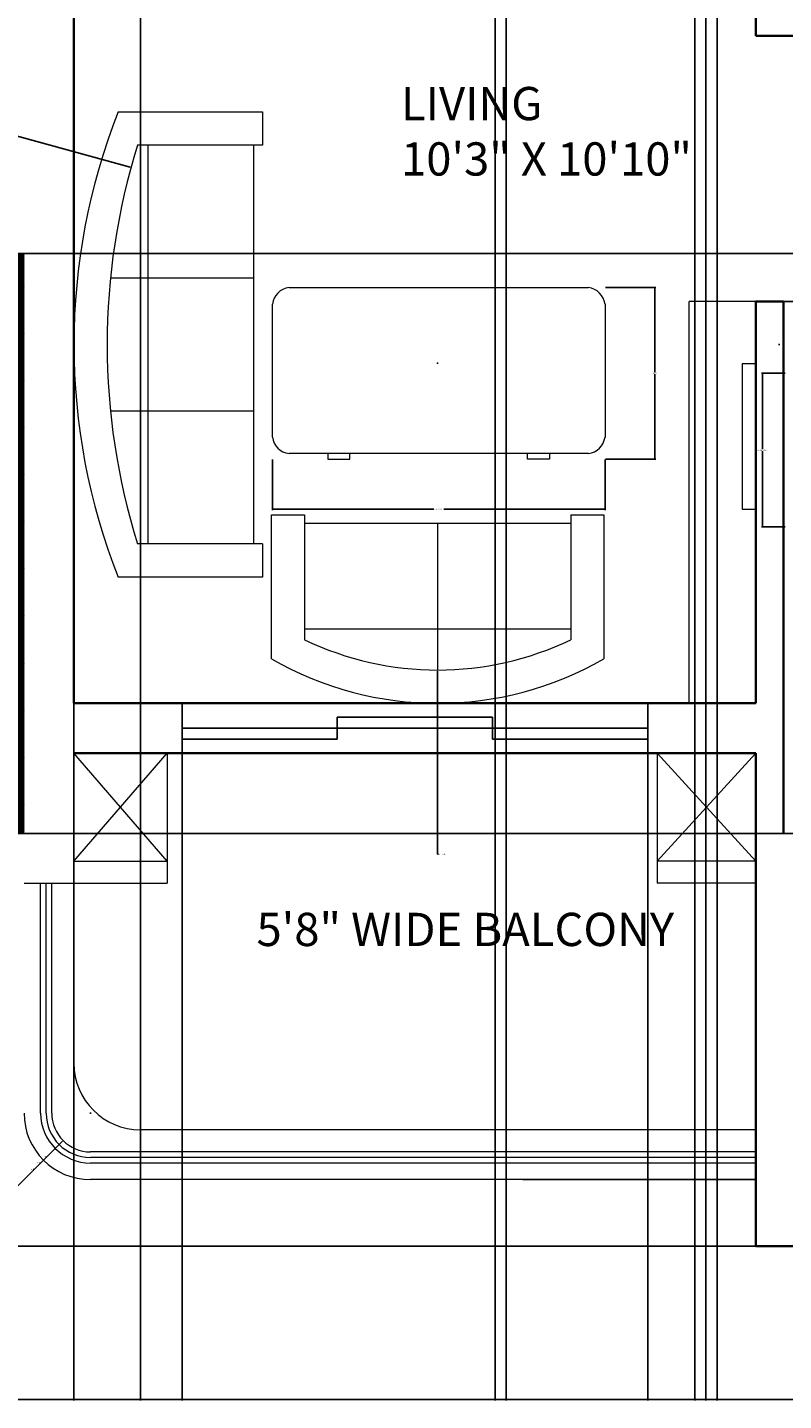
# Model space of a CAD drawing. Units: inches. Extents: x 6662 to 7211, y 5077 to 5683.
# Tile 3 of 9: x 6870 to 7007, y 5077 to 5325. Entities that reach past the tile are written whole.
import ezdxf

# ---------------------------------------------------------------- set-up
doc = ezdxf.new("R2010")
doc.units = ezdxf.units.IN
doc.header["$LTSCALE"] = 3
doc.header["$MEASUREMENT"] = 0
for name, color, linetype, lineweight in [('A-ANNO-DIMS', 2, 'Continuous', 18), ('A-AREA-IDEN', 7, 'Continuous', 18), ('A-DOOR', 4, 'Continuous', 25), ('A-EQPM', 8, 'Continuous', 18), ('A-FLOR-CASE', 8, 'Continuous', 20), ('A-FLOR-CASE-PATT', 241, 'Continuous', 13), ('A-FLOR-HRAL', 7, 'Continuous', 18), ('A-FLOR-PROJ', 7, 'Continuous', 18), ('A-FURN', 8, 'Continuous', 18), ('A-WALL', 7, 'Continuous', 35)]:
    doc.layers.add(name, color=color, linetype=linetype, lineweight=lineweight)
doc.styles.get("Standard").update_dxf_attribs({"font": 'arial.ttf'})
doc.dimstyles.get("Standard").update_dxf_attribs({"dimtxt": 0.18, "dimasz": 0.18, "dimexe": 0.18, "dimexo": 0.0625, "dimgap": 0.09, "dimtad": 0, "dimtih": 1, "dimtoh": 1, "dimdec": 4, "dimzin": 0, "dimdsep": 46, "dimtxsty": 'Standard', "dimcen": 0.09, "dimadec": 0, "dimazin": 0, "dimtfac": 1, "dimtdec": 4, "dimtofl": 0, "dimtmove": 0, "dimatfit": 3, "dimfxl": 1, "dimtolj": 1, "dimtzin": 0, "dimarcsym": 0})

# ---------------------------------------------------------------- blocks, each defined once
blk = doc.blocks.new('Sofa - Roundback 7 ft.')
for p, q in [((-12.00002, -32.4421), (-12.00003, -6.5971)), ((11.99997, -32.4421), (11.99998, -6.5971)), ((-36.000027, -34), (-36.000027, -11.4696)), ((35.99998, -34), (35.99998, -11.4696)), ((-35.999844, -13.3819), (35.9998, -13.3819)), ((-36.000027, -32.4421), (35.99998, -32.4421))]:
    blk.add_line(p, q)
for points in [[(-36.000027, -34), (-42.000027, -34), (-42.000027, -8)], [(41.99998, -8), (41.99998, -34), (35.99998, -34)]]:
    blk.add_lwpolyline(points)
for centre, radius, start, end in [((0, -114.25), 114.25, 68.43141, 111.5686), ((-0.00001, -127.1968), 121.1968, 72.72033, 107.2797)]:
    blk.add_arc(centre, radius, start, end)
blk = doc.blocks.new('Desk - 30 x 60 in.')
for p, q in [((-26.999995, 0), (26.999995, 0)), ((-29.999995, -27), (-29.999995, -3)), ((29.999995, -3), (29.999995, -27)), ((26.999995, -30), (-26.999995, -30)), ((-20.000005, -30), (-20.000005, -31)), ((-20.000005, -31), (-16.000005, -31)), ((-16.000005, -31), (-16.000005, -30)), ((15.999995, -31), (15.999995, -30)), ((19.999995, -31), (15.999995, -31)), ((19.999995, -30), (19.999995, -31))]:
    blk.add_line(p, q)
for centre, start, end in [((-26.499995, -3.5), 98.1301, 171.8699), ((26.499995, -3.5), 8.130102, 81.8699), ((-26.499995, -26.5), 188.1301, 261.8699), ((26.499995, -26.5), 278.1301, 351.8699)]:
    blk.add_arc(centre, 3.535534, start, end)
blk = doc.blocks.new('Sofa - Roundback Loveseat 5 ft.')
for p, q in [((0, -32.44198), (0, -5.99998)), ((-24, -33.99998), (-24, -11.46958)), ((24.00004, -33.99998), (24.00004, -11.46958)), ((-23.9998, -13.38178), (23.99986, -13.38178)), ((-24, -32.44198), (24.00004, -32.44198))]:
    blk.add_line(p, q)
for points in [[(-24, -33.99998), (-30, -33.99998), (-30, -7.99998)], [(30.00004, -7.99998), (30.00004, -33.99998), (24.00004, -33.99998)]]:
    blk.add_lwpolyline(points)
for centre, radius, start, end in [((0, -60.24998), 60.24998, 60.13715, 119.8628), ((0, -61.38438), 55.38444, 64.32083, 115.6792)]:
    blk.add_arc(centre, radius, start, end)
blk = doc.blocks.new('*D30')
at = {"layer": 'A-ANNO-DIMS', "color": 0, "lineweight": -2, "ltscale": 3, "transparency": 16777216}
for p, q in [((6914.66, 5246.6), (6914.66, 5237.48)), ((6974.66, 5246.6), (6974.66, 5237.48)), ((6914.84, 5237.66), (6943.76, 5237.66)), ((6974.48, 5237.66), (6945.56, 5237.66))]:
    blk.add_line(p, q, dxfattribs=at)
at = {"layer": 'A-ANNO-DIMS', "color": 0, "ltscale": 3, "transparency": 16777216}
for points in [[(6914.84, 5237.69), (6914.84, 5237.63), (6914.66, 5237.66)], [(6974.48, 5237.69), (6974.48, 5237.63), (6974.66, 5237.66)]]:
    blk.add_solid(points, dxfattribs=at)
at = {"layer": 'Defpoints', "color": 0, "ltscale": 3, "transparency": 16777216}
for p in [(6914.66, 5246.66), (6974.66, 5246.66), (6974.66, 5237.66)]:
    blk.add_point(p, dxfattribs=at)
at = {"layer": 'A-ANNO-DIMS', "color": 0, "ltscale": 3, "transparency": 16777216, "insert": (6944.66, 5237.66), "char_height": 0.18, "attachment_point": 5}
blk.add_mtext('\\A1;DESK 60 TYP.', dxfattribs=at)
blk = doc.blocks.new('*D31')
at = {"layer": 'A-ANNO-DIMS', "color": 0, "lineweight": -2, "ltscale": 3, "transparency": 16777216}
for p, q in [((6974.72, 5277.66), (6983.84, 5277.66)), ((6983.66, 5277.48), (6983.66, 5262.34)), ((6983.66, 5246.84), (6983.66, 5261.98)), ((6974.72, 5246.66), (6983.84, 5246.66))]:
    blk.add_line(p, q, dxfattribs=at)
at = {"layer": 'A-ANNO-DIMS', "color": 0, "ltscale": 3, "transparency": 16777216}
for points in [[(6983.63, 5277.48), (6983.69, 5277.48), (6983.66, 5277.66)], [(6983.63, 5246.84), (6983.69, 5246.84), (6983.66, 5246.66)]]:
    blk.add_solid(points, dxfattribs=at)
at = {"layer": 'Defpoints', "color": 0, "ltscale": 3, "transparency": 16777216}
for p in [(6974.66, 5277.66), (6983.66, 5277.66), (6974.66, 5246.66)]:
    blk.add_point(p, dxfattribs=at)
at = {"layer": 'A-ANNO-DIMS', "color": 0, "ltscale": 3, "transparency": 16777216, "insert": (6983.66, 5262.16), "char_height": 0.18, "attachment_point": 5}
blk.add_mtext('\\A1;31 TYP.', dxfattribs=at)
blk = doc.blocks.new('*D36')
at = {"layer": 'A-ANNO-DIMS', "color": 0, "lineweight": -2, "ltscale": 3, "transparency": 16777216}
for p, q in [((7007.15, 5262.16), (7002.88, 5262.16)), ((7003.06, 5261.98), (7003.06, 5248.48)), ((7003.06, 5234.61), (7003.06, 5248.11)), ((7007.15, 5234.43), (7002.88, 5234.43))]:
    blk.add_line(p, q, dxfattribs=at)
at = {"layer": 'A-ANNO-DIMS', "color": 0, "ltscale": 3, "transparency": 16777216}
for points in [[(7003.03, 5261.98), (7003.09, 5261.98), (7003.06, 5262.16)], [(7003.03, 5234.61), (7003.09, 5234.61), (7003.06, 5234.43)]]:
    blk.add_solid(points, dxfattribs=at)
at = {"layer": 'Defpoints', "color": 0, "ltscale": 3, "transparency": 16777216}
for p in [(7007.22, 5262.16), (7003.06, 5234.43), (7007.22, 5234.43)]:
    blk.add_point(p, dxfattribs=at)
at = {"layer": 'A-ANNO-DIMS', "color": 0, "ltscale": 3, "transparency": 16777216, "insert": (7003.06, 5248.29), "char_height": 0.18, "attachment_point": 5}
blk.add_mtext('\\A1;REFRIGERATOR 28', dxfattribs=at)
blk = doc.blocks.new('*D40')
at = {"layer": 'A-ANNO-DIMS', "color": 0, "lineweight": -2, "ltscale": 3, "transparency": 16777216}
for p, q in [((7182.86, 5326.04), (7182.86, 5076.72)), ((6689.86, 5323.04), (6689.86, 5076.72)), ((6690.04, 5076.9), (6936.07, 5076.9)), ((7182.68, 5076.9), (6936.65, 5076.9))]:
    blk.add_line(p, q, dxfattribs=at)
at = {"layer": 'A-ANNO-DIMS', "color": 0, "ltscale": 3, "transparency": 16777216}
for points in [[(6690.04, 5076.93), (6690.04, 5076.87), (6689.86, 5076.9)], [(7182.68, 5076.93), (7182.68, 5076.87), (7182.86, 5076.9)]]:
    blk.add_solid(points, dxfattribs=at)
at = {"layer": 'Defpoints', "color": 0, "ltscale": 3, "transparency": 16777216}
for p in [(7182.86, 5326.1), (6689.86, 5323.1), (7182.86, 5076.9)]:
    blk.add_point(p, dxfattribs=at)
at = {"layer": 'A-ANNO-DIMS', "color": 0, "ltscale": 3, "transparency": 16777216, "insert": (6936.36, 5076.9), "char_height": 0.18, "attachment_point": 5}
blk.add_mtext('\\A1;493', dxfattribs=at)
blk = doc.blocks.new('*D60')
at = {"layer": 'A-ANNO-DIMS', "color": 0, "lineweight": -2, "ltscale": 3, "transparency": 16777216}
for p, q in [((6716.8, 5170.1), (6661.98, 5170.1)), ((6662.16, 5169.92), (6662.16, 5137.53)), ((6662.16, 5104.78), (6662.16, 5137.17)), ((7001.8, 5104.6), (6661.98, 5104.6))]:
    blk.add_line(p, q, dxfattribs=at)
at = {"layer": 'A-ANNO-DIMS', "color": 0, "ltscale": 3, "transparency": 16777216}
for points in [[(6662.13, 5169.92), (6662.19, 5169.92), (6662.16, 5170.1)], [(6662.13, 5104.78), (6662.19, 5104.78), (6662.16, 5104.6)]]:
    blk.add_solid(points, dxfattribs=at)
at = {"layer": 'Defpoints', "color": 0, "ltscale": 3, "transparency": 16777216}
for p in [(6716.86, 5170.1), (6662.16, 5104.6), (7001.86, 5104.6)]:
    blk.add_point(p, dxfattribs=at)
at = {"layer": 'A-ANNO-DIMS', "color": 0, "ltscale": 3, "transparency": 16777216, "insert": (6662.16, 5137.35), "char_height": 0.18, "attachment_point": 5}
blk.add_mtext('\\A1;65.5', dxfattribs=at)
blk = doc.blocks.new('*D66')
at = {"layer": 'A-ANNO-DIMS', "color": 0, "lineweight": -2, "ltscale": 3, "transparency": 16777216}
for p, q in [((6956.86, 5464.54), (6956.86, 5076.72)), ((6992.86, 5464.54), (6992.86, 5076.72)), ((6957.04, 5076.9), (6974.64, 5076.9)), ((6992.68, 5076.9), (6975.08, 5076.9))]:
    blk.add_line(p, q, dxfattribs=at)
at = {"layer": 'A-ANNO-DIMS', "color": 0, "ltscale": 3, "transparency": 16777216}
for points in [[(6957.04, 5076.93), (6957.04, 5076.87), (6956.86, 5076.9)], [(6992.68, 5076.93), (6992.68, 5076.87), (6992.86, 5076.9)]]:
    blk.add_solid(points, dxfattribs=at)
at = {"layer": 'Defpoints', "color": 0, "ltscale": 3, "transparency": 16777216}
for p in [(6956.86, 5464.6), (6992.86, 5464.6), (6992.86, 5076.9)]:
    blk.add_point(p, dxfattribs=at)
at = {"layer": 'A-ANNO-DIMS', "color": 0, "ltscale": 3, "transparency": 16777216, "insert": (6974.86, 5076.9), "char_height": 0.18, "attachment_point": 5}
blk.add_mtext('\\A1;36', dxfattribs=at)
blk = doc.blocks.new('*D67')
at = {"layer": 'A-ANNO-DIMS', "color": 0, "lineweight": -2, "ltscale": 3, "transparency": 16777216}
for p, q in [((6994.86, 5514.54), (6994.86, 5076.72)), ((7024.86, 5514.54), (7024.86, 5076.72)), ((6995.04, 5076.9), (7009.64, 5076.9)), ((7024.68, 5076.9), (7010.08, 5076.9))]:
    blk.add_line(p, q, dxfattribs=at)
at = {"layer": 'A-ANNO-DIMS', "color": 0, "ltscale": 3, "transparency": 16777216}
for points in [[(6995.04, 5076.93), (6995.04, 5076.87), (6994.86, 5076.9)], [(7024.68, 5076.93), (7024.68, 5076.87), (7024.86, 5076.9)]]:
    blk.add_solid(points, dxfattribs=at)
at = {"layer": 'Defpoints', "color": 0, "ltscale": 3, "transparency": 16777216}
for p in [(6994.86, 5514.6), (7024.86, 5514.6), (7024.86, 5076.9)]:
    blk.add_point(p, dxfattribs=at)
at = {"layer": 'A-ANNO-DIMS', "color": 0, "ltscale": 3, "transparency": 16777216, "insert": (7009.86, 5076.9), "char_height": 0.18, "attachment_point": 5}
blk.add_mtext('\\A1;30', dxfattribs=at)
blk = doc.blocks.new('*D70')
at = {"layer": 'A-ANNO-DIMS', "color": 0, "lineweight": -2, "ltscale": 3, "transparency": 16777216}
for p, q in [((6898.36, 5193.54), (6898.36, 5076.72)), ((6982.36, 5193.54), (6982.36, 5076.72)), ((6898.54, 5076.9), (6940.14, 5076.9)), ((6982.18, 5076.9), (6940.58, 5076.9))]:
    blk.add_line(p, q, dxfattribs=at)
at = {"layer": 'A-ANNO-DIMS', "color": 0, "ltscale": 3, "transparency": 16777216}
for points in [[(6898.54, 5076.93), (6898.54, 5076.87), (6898.36, 5076.9)], [(6982.18, 5076.93), (6982.18, 5076.87), (6982.36, 5076.9)]]:
    blk.add_solid(points, dxfattribs=at)
at = {"layer": 'Defpoints', "color": 0, "ltscale": 3, "transparency": 16777216}
for p in [(6898.36, 5193.6), (6982.36, 5193.6), (6982.36, 5076.9)]:
    blk.add_point(p, dxfattribs=at)
at = {"layer": 'A-ANNO-DIMS', "color": 0, "ltscale": 3, "transparency": 16777216, "insert": (6940.36, 5076.9), "char_height": 0.18, "attachment_point": 5}
blk.add_mtext('\\A1;84', dxfattribs=at)
blk = doc.blocks.new('*D71')
at = {"layer": 'A-ANNO-DIMS', "color": 0, "lineweight": -2, "ltscale": 3, "transparency": 16777216}
for p, q in [((6878.86, 5617.54), (6878.86, 5076.72)), ((6890.86, 5617.54), (6890.86, 5076.72)), ((6879.04, 5076.9), (6884.65, 5076.9)), ((6890.68, 5076.9), (6885.07, 5076.9))]:
    blk.add_line(p, q, dxfattribs=at)
at = {"layer": 'A-ANNO-DIMS', "color": 0, "ltscale": 3, "transparency": 16777216}
for points in [[(6879.04, 5076.93), (6879.04, 5076.87), (6878.86, 5076.9)], [(6890.68, 5076.93), (6890.68, 5076.87), (6890.86, 5076.9)]]:
    blk.add_solid(points, dxfattribs=at)
at = {"layer": 'Defpoints', "color": 0, "ltscale": 3, "transparency": 16777216}
for p in [(6878.86, 5617.6), (6890.86, 5617.6), (6878.86, 5076.9)]:
    blk.add_point(p, dxfattribs=at)
at = {"layer": 'A-ANNO-DIMS', "color": 0, "ltscale": 3, "transparency": 16777216, "insert": (6884.86, 5076.9), "char_height": 0.18, "attachment_point": 5}
blk.add_mtext('\\A1;12', dxfattribs=at)
blk = doc.blocks.new('*D72')
at = {"layer": 'A-ANNO-DIMS', "color": 0, "lineweight": -2, "ltscale": 3, "transparency": 16777216}
for p, q in [((6954.86, 5617.54), (6954.86, 5076.72)), ((6990.86, 5617.54), (6990.86, 5076.72)), ((6955.04, 5076.9), (6972.64, 5076.9)), ((6990.68, 5076.9), (6973.08, 5076.9))]:
    blk.add_line(p, q, dxfattribs=at)
at = {"layer": 'A-ANNO-DIMS', "color": 0, "ltscale": 3, "transparency": 16777216}
for points in [[(6955.04, 5076.93), (6955.04, 5076.87), (6954.86, 5076.9)], [(6990.68, 5076.93), (6990.68, 5076.87), (6990.86, 5076.9)]]:
    blk.add_solid(points, dxfattribs=at)
at = {"layer": 'Defpoints', "color": 0, "ltscale": 3, "transparency": 16777216}
for p in [(6954.86, 5617.6), (6990.86, 5617.6), (6990.86, 5076.9)]:
    blk.add_point(p, dxfattribs=at)
at = {"layer": 'A-ANNO-DIMS', "color": 0, "ltscale": 3, "transparency": 16777216, "insert": (6972.86, 5076.9), "char_height": 0.18, "attachment_point": 5}
blk.add_mtext('\\A1;36', dxfattribs=at)
blk = doc.blocks.new('*D78')
at = {"layer": 'A-ANNO-DIMS', "color": 0, "lineweight": -2, "ltscale": 3, "transparency": 16777216}
for p, q in [((7001.92, 5323.1), (7210.74, 5323.1)), ((7210.56, 5322.92), (7210.56, 5299.28)), ((7210.56, 5275.28), (7210.56, 5298.92)), ((7006.92, 5275.1), (7210.74, 5275.1))]:
    blk.add_line(p, q, dxfattribs=at)
at = {"layer": 'A-ANNO-DIMS', "color": 0, "ltscale": 3, "transparency": 16777216}
for points in [[(7210.53, 5322.92), (7210.59, 5322.92), (7210.56, 5323.1)], [(7210.53, 5275.28), (7210.59, 5275.28), (7210.56, 5275.1)]]:
    blk.add_solid(points, dxfattribs=at)
at = {"layer": 'Defpoints', "color": 0, "ltscale": 3, "transparency": 16777216}
for p in [(7001.86, 5323.1), (7210.56, 5323.1), (7006.86, 5275.1)]:
    blk.add_point(p, dxfattribs=at)
at = {"layer": 'A-ANNO-DIMS', "color": 0, "ltscale": 3, "transparency": 16777216, "insert": (7210.56, 5299.1), "char_height": 0.18, "attachment_point": 5}
blk.add_mtext('\\A1;48', dxfattribs=at)
blk = doc.blocks.new('*D83')
at = {"layer": 'A-ANNO-DIMS', "color": 0, "lineweight": -2, "ltscale": 3, "transparency": 16777216}
for p, q in [((6845.92, 5283.8), (7210.74, 5283.8)), ((7210.56, 5283.62), (7210.56, 5231.63)), ((7210.56, 5179.28), (7210.56, 5231.27)), ((6845.92, 5179.1), (7210.74, 5179.1))]:
    blk.add_line(p, q, dxfattribs=at)
at = {"layer": 'A-ANNO-DIMS', "color": 0, "ltscale": 3, "transparency": 16777216}
for points in [[(7210.53, 5283.62), (7210.59, 5283.62), (7210.56, 5283.8)], [(7210.53, 5179.28), (7210.59, 5179.28), (7210.56, 5179.1)]]:
    blk.add_solid(points, dxfattribs=at)
at = {"layer": 'Defpoints', "color": 0, "ltscale": 3, "transparency": 16777216}
for p in [(6845.86, 5283.8), (7210.56, 5283.8), (6845.86, 5179.1)]:
    blk.add_point(p, dxfattribs=at)
at = {"layer": 'A-ANNO-DIMS', "color": 0, "ltscale": 3, "transparency": 16777216, "insert": (7210.56, 5231.45), "char_height": 0.18, "attachment_point": 5}
blk.add_mtext('\\A1;104.7', dxfattribs=at)
blk = doc.blocks.new('*D87')
at = {"layer": 'A-ANNO-DIMS', "color": 0, "lineweight": -2, "ltscale": 3, "transparency": 16777216}
for p, q in [((6881.86, 5128.51), (6881.86, 5128.69)), ((6881.77, 5128.6), (6881.95, 5128.6)), ((6868.28, 5115.02), (6873.25, 5119.99)), ((6868.1, 5115.02), (6868.28, 5115.02))]:
    blk.add_line(p, q, dxfattribs=at)
at = {"layer": 'A-ANNO-DIMS', "color": 0, "ltscale": 3, "transparency": 16777216}
blk.add_solid([(6873.22, 5120.01), (6873.27, 5119.96), (6873.37, 5120.11)], dxfattribs=at)
at = {"layer": 'Defpoints', "color": 0, "ltscale": 3, "transparency": 16777216}
for p in [(6881.86, 5128.6), (6873.37, 5120.11)]:
    blk.add_point(p, dxfattribs=at)
at = {"layer": 'A-ANNO-DIMS', "color": 0, "ltscale": 3, "transparency": 16777216, "insert": (6867.6, 5115.02), "char_height": 0.18, "attachment_point": 5}
blk.add_mtext('\\A1;2X R12', dxfattribs=at)
blk = doc.blocks.new('*D96')
at = {"layer": 'A-ANNO-DIMS', "color": 0, "lineweight": -2, "ltscale": 3, "transparency": 16777216}
for p, q in [((6881.86, 5128.51), (6881.86, 5128.69)), ((6881.77, 5128.6), (6881.95, 5128.6)), ((6871.68, 5118.42), (6875.37, 5122.11)), ((6871.5, 5118.42), (6871.68, 5118.42))]:
    blk.add_line(p, q, dxfattribs=at)
at = {"layer": 'A-ANNO-DIMS', "color": 0, "ltscale": 3, "transparency": 16777216}
blk.add_solid([(6875.35, 5122.13), (6875.39, 5122.09), (6875.49, 5122.23)], dxfattribs=at)
at = {"layer": 'Defpoints', "color": 0, "ltscale": 3, "transparency": 16777216}
for p in [(6881.86, 5128.6), (6875.49, 5122.23)]:
    blk.add_point(p, dxfattribs=at)
at = {"layer": 'A-ANNO-DIMS', "color": 0, "ltscale": 3, "transparency": 16777216, "insert": (6871.26, 5118.42), "char_height": 0.18, "attachment_point": 5}
blk.add_mtext('\\A1;R9', dxfattribs=at)
blk = doc.blocks.new('*D97')
at = {"layer": 'A-ANNO-DIMS', "color": 0, "lineweight": -2, "ltscale": 3, "transparency": 16777216}
for p, q in [((6881.86, 5128.51), (6881.86, 5128.69)), ((6881.77, 5128.6), (6881.95, 5128.6)), ((6872.81, 5119.55), (6876.07, 5122.81)), ((6872.63, 5119.55), (6872.81, 5119.55))]:
    blk.add_line(p, q, dxfattribs=at)
at = {"layer": 'A-ANNO-DIMS', "color": 0, "ltscale": 3, "transparency": 16777216}
blk.add_solid([(6876.05, 5122.83), (6876.09, 5122.79), (6876.2, 5122.94)], dxfattribs=at)
at = {"layer": 'Defpoints', "color": 0, "ltscale": 3, "transparency": 16777216}
for p in [(6881.86, 5128.6), (6876.2, 5122.94)]:
    blk.add_point(p, dxfattribs=at)
at = {"layer": 'A-ANNO-DIMS', "color": 0, "ltscale": 3, "transparency": 16777216, "insert": (6872.39, 5119.55), "char_height": 0.18, "attachment_point": 5}
blk.add_mtext('\\A1;R8', dxfattribs=at)
blk = doc.blocks.new('*D98')
at = {"layer": 'A-ANNO-DIMS', "color": 0, "lineweight": -2, "ltscale": 3, "transparency": 16777216}
for p, q in [((6881.86, 5128.51), (6881.86, 5128.69)), ((6881.77, 5128.6), (6881.95, 5128.6)), ((6873.94, 5120.68), (6876.78, 5123.52)), ((6873.76, 5120.68), (6873.94, 5120.68))]:
    blk.add_line(p, q, dxfattribs=at)
at = {"layer": 'A-ANNO-DIMS', "color": 0, "ltscale": 3, "transparency": 16777216}
blk.add_solid([(6876.76, 5123.54), (6876.8, 5123.5), (6876.91, 5123.65)], dxfattribs=at)
at = {"layer": 'Defpoints', "color": 0, "ltscale": 3, "transparency": 16777216}
for p in [(6881.86, 5128.6), (6876.91, 5123.65)]:
    blk.add_point(p, dxfattribs=at)
at = {"layer": 'A-ANNO-DIMS', "color": 0, "ltscale": 3, "transparency": 16777216, "insert": (6873.52, 5120.68), "char_height": 0.18, "attachment_point": 5}
blk.add_mtext('\\A1;R7', dxfattribs=at)
blk = doc.blocks.new('*D100')
at = {"layer": 'A-ANNO-DIMS', "color": 0, "lineweight": -2, "ltscale": 3, "transparency": 16777216}
for p, q in [((6818.84, 5318.55), (6819.02, 5318.55)), ((6819.02, 5318.55), (6888.99, 5299.4)), ((7005.96, 5267.35), (7006.14, 5267.35)), ((7006.05, 5267.26), (7006.05, 5267.44))]:
    blk.add_line(p, q, dxfattribs=at)
at = {"layer": 'A-ANNO-DIMS', "color": 0, "ltscale": 3, "transparency": 16777216}
blk.add_solid([(6888.99, 5299.43), (6888.98, 5299.37), (6889.16, 5299.35)], dxfattribs=at)
at = {"layer": 'Defpoints', "color": 0, "ltscale": 3, "transparency": 16777216}
for p in [(6889.16, 5299.35), (7006.05, 5267.35)]:
    blk.add_point(p, dxfattribs=at)
at = {"layer": 'A-ANNO-DIMS', "color": 0, "ltscale": 3, "transparency": 16777216, "insert": (6818.17, 5318.55), "char_height": 0.18, "attachment_point": 5}
blk.add_mtext('\\A1;2X R121.2', dxfattribs=at)
blk = doc.blocks.new('*D104')
at = {"layer": 'A-ANNO-DIMS', "color": 0, "lineweight": -2, "ltscale": 3, "transparency": 16777216}
for p, q in [((6944.38, 5263.98), (6944.56, 5263.98)), ((6944.47, 5263.89), (6944.47, 5264.07)), ((6944.47, 5175.37), (6944.47, 5208.42)), ((6944.65, 5175.37), (6944.47, 5175.37))]:
    blk.add_line(p, q, dxfattribs=at)
at = {"layer": 'A-ANNO-DIMS', "color": 0, "ltscale": 3, "transparency": 16777216}
blk.add_solid([(6944.5, 5208.42), (6944.44, 5208.42), (6944.47, 5208.6)], dxfattribs=at)
at = {"layer": 'Defpoints', "color": 0, "ltscale": 3, "transparency": 16777216}
for p in [(6944.47, 5263.98), (6944.47, 5208.6)]:
    blk.add_point(p, dxfattribs=at)
at = {"layer": 'A-ANNO-DIMS', "color": 0, "ltscale": 3, "transparency": 16777216, "insert": (6945.33, 5175.37), "char_height": 0.18, "attachment_point": 5}
blk.add_mtext('\\A1;2X R55.38', dxfattribs=at)

msp = doc.modelspace()

# ---------------------------------------------------------------- hatches: boundary and pattern name
at = {"layer": 'A-FLOR-CASE-PATT'}
h = msp.add_hatch(dxfattribs=at)
h.set_pattern_fill('ANSI31', color=256)
h.paths.add_polyline_path([(6869.8579, 5283.7981), (6845.8579, 5283.7981), (6845.8579, 5229.4653), (6847.018, 5229.7817, -0.54116316), (6849.0925, 5228.1371), (6849.7129, 5228.234, -0.50821327), (6851.018, 5227.2817), (6851.018, 5226.7817), (6855.018, 5227.2817), (6855.018, 5225.7817), (6851.018, 5225.2817), (6851.018, 5217.7817), (6851.018, 5210.2817), (6855.018, 5209.7817), (6855.018, 5208.2817), (6851.018, 5208.7817), (6851.018, 5208.2817, -0.41421356), (6850.018, 5207.2817), (6849.0925, 5207.4263, -0.50580924), (6847.1872, 5205.7355), (6845.8579, 5206.0981), (6845.8579, 5179.0979), (6869.8579, 5179.0979)])
h.paths.add_polyline_path([(7167.8579, 5497.5979), (7143.8579, 5497.5979), (7078.3579, 5497.5979), (7078.3579, 5473.5979), (7163.8579, 5473.5979), (7167.8579, 5473.5979)])
h.paths.add_polyline_path([(6825.9016, 5497.5979), (6725.8579, 5497.5979), (6725.8579, 5473.5979), (6825.9016, 5473.5979)])
h.paths.add_polyline_path([(6796.6359, 5485.2095), (6797.1359, 5489.2095), (6806.1359, 5489.2095), (6815.1359, 5489.2095), (6815.6359, 5485.2095), (6814.1359, 5485.2095), (6813.6359, 5489.2095), (6806.1359, 5489.2095), (6798.6359, 5489.2095), (6798.1359, 5485.2095)], flags=16)

# ---------------------------------------------------------------- linework, layer by layer
at = {"layer": 'A-DOOR'}
for p, q in [((6898.3579, 5193.5979), (6898.3579, 5202.5979)), ((6982.3579, 5193.5979), (6982.3579, 5202.5979)), ((6898.3579, 5198.0979), (6982.3579, 5198.0979)), ((6926.3579, 5200.0979), (6954.3579, 5200.0979)), ((6926.3579, 5200.0979), (6926.3579, 5196.0979)), ((6954.3579, 5200.0979), (6954.3579, 5196.0979)), ((6898.3579, 5196.0979), (6926.3579, 5196.0979)), ((6954.3579, 5196.0979), (6982.3579, 5196.0979))]:
    msp.add_line(p, q, dxfattribs=at)
at = {"layer": 'A-EQPM'}
msp.add_lwpolyline([(7001.8579, 5263.8505), (6999.3887, 5263.8505), (6999.3887, 5237.6131), (7001.8579, 5237.6131)], close=True, dxfattribs=at)
at = {"layer": 'A-FLOR-CASE'}
for p in [(6989.8579, 5202.5979), (7001.8579, 5275.0979)]:
    msp.add_line(p, (6989.8579, 5275.0979), dxfattribs=at)
at = {"layer": 'A-FLOR-HRAL'}
for p, q in [((6878.8579, 5137.5979), (6878.8579, 5193.5979)), ((6878.8579, 5170.0979), (6878.8579, 5193.5979)), ((6869.8579, 5170.0979), (6878.8579, 5170.0979)), ((6872.8579, 5128.5979), (6872.8579, 5170.0979)), ((6873.8579, 5128.5979), (6873.8579, 5170.0979)), ((6874.8579, 5128.5979), (6874.8579, 5170.0979)), ((7001.8579, 5125.5979), (6890.8579, 5125.5979)), ((7001.8579, 5121.5979), (6881.8579, 5121.5979)), ((7001.8579, 5120.5979), (6881.8579, 5120.5979)), ((7001.8579, 5119.5979), (6881.8579, 5119.5979)), ((7001.8579, 5116.5979), (6881.8579, 5116.5979)), ((6959.8579, 5116.5979), (7001.8579, 5116.5979))]:
    msp.add_line(p, q, dxfattribs=at)
for centre, radius in [((6890.8579, 5137.5979), 12), ((6881.8579, 5128.5979), 12), ((6881.8579, 5128.5979), 9), ((6881.8579, 5128.5979), 8), ((6881.8579, 5128.5979), 7)]:
    msp.add_arc(centre, radius, 180, 270, dxfattribs=at)
at = {"layer": 'A-FLOR-PROJ'}
for p, q in [((6895.6735, 5174.0979), (6878.8579, 5193.5979)), ((6878.8579, 5174.0979), (6895.6735, 5193.5979)), ((6895.6735, 5193.5979), (6895.6735, 5170.0979)), ((6984.0475, 5193.5979), (6984.0475, 5170.0979)), ((7001.8579, 5193.5979), (6984.0475, 5174.0979)), ((6984.0475, 5193.5979), (7001.8579, 5174.0979)), ((6878.8579, 5174.0979), (6895.6735, 5174.0979)), ((7001.8579, 5174.0979), (6984.0475, 5174.0979)), ((6878.8579, 5170.0979), (6895.6735, 5170.0979)), ((7001.8579, 5170.0979), (6984.0475, 5170.0979))]:
    msp.add_line(p, q, dxfattribs=at)
at = {"layer": 'A-WALL'}
for p, q in [((6878.8579, 5202.5979), (6878.8579, 5332.0979)), ((7001.8579, 5323.0979), (7001.8579, 5332.0979)), ((7001.8579, 5323.0979), (7001.8579, 5332.0979)), ((7006.8579, 5323.0979), (7001.8579, 5323.0979)), ((7102.8579, 5323.0979), (7006.8579, 5323.0979)), ((7001.8579, 5202.5979), (7001.8579, 5275.0979)), ((7001.8579, 5202.5979), (7001.8579, 5275.0979)), ((7006.8579, 5275.0979), (7001.8579, 5275.0979)), ((7006.8579, 5179.0979), (7006.8579, 5275.0979)), ((7001.8579, 5202.5979), (6878.8579, 5202.5979)), ((7001.8579, 5193.5979), (6878.8579, 5193.5979)), ((7001.8579, 5125.5979), (7001.8579, 5193.5979)), ((7001.8579, 5116.5979), (7001.8579, 5125.5979)), ((7001.8579, 5104.5979), (7001.8579, 5116.5979)), ((7010.8579, 5104.5979), (7001.8579, 5104.5979))]:
    msp.add_line(p, q, dxfattribs=at)

# ---------------------------------------------------------------- block references
at = {"layer": 'A-FURN'}
for name, p, rotation in [('Sofa - Roundback 7 ft.', (6878.8579, 5267.3479), 90), ('Sofa - Roundback Loveseat 5 ft.', (6944.4736, 5202.5979), 180)]:
    msp.add_blockref(name, p, dxfattribs=dict(at, rotation=rotation))
msp.add_blockref('Desk - 30 x 60 in.', (6944.6609, 5277.6598), dxfattribs=at)

# ---------------------------------------------------------------- texts
at = {"layer": 'A-AREA-IDEN', "ltscale": 3, "char_height": 6, "attachment_point": 1}
for s, insert in [('LIVING\\P10\'3" X 10\'10"', (6937.8737, 5313.8611)), ('5\'8" WIDE BALCONY', (6911.7969, 5164.7703))]:
    msp.add_mtext_dynamic_manual_height_columns(s, width=381.547883, gutter_width=1, heights=[0], dxfattribs=dict(at, insert=insert))

# ---------------------------------------------------------------- dimensions: what is measured, and where the dimension line sits
at = {"layer": 'A-ANNO-DIMS', "ltscale": 3}
for base, p1, p2, picture, middle in [((6878.8579, 5076.8979), (6890.8579, 5617.5979), (6878.8579, 5617.5979), '*D71', (6884.8579, 5076.8979)), ((6990.8579, 5076.8979), (6954.8579, 5617.5979), (6990.8579, 5617.5979), '*D72', (6972.8579, 5076.8979)), ((7024.8579, 5076.8979), (6994.8579, 5514.5979), (7024.8579, 5514.5979), '*D67', (7009.8579, 5076.8979)), ((6992.8579, 5076.8979), (6956.8579, 5464.5979), (6992.8579, 5464.5979), '*D66', (6974.8579, 5076.8979)), ((7182.8579, 5076.8979), (6689.8579, 5323.0979), (7182.8579, 5326.0979), '*D40', (6936.3579, 5076.8979)), ((6982.3579, 5076.8979), (6898.3579, 5193.5979), (6982.3579, 5193.5979), '*D70', (6940.3579, 5076.8979))]:
    dim = msp.add_linear_dim(base=base, p1=p1, p2=p2, dimstyle='Standard', override={"dimdec": 0, "dimlfac": 1, "dimrnd": 0, "dimzin": 0, "dimdsep": 46, "dimlunit": 2}, dxfattribs=at)
    dim.commit()
    dim.dimension.update_dxf_attribs({"geometry": picture, "text_midpoint": middle})
for base, p1, p2, override, picture, middle in [((7210.5579, 5323.0979), (7006.8579, 5275.0979), (7001.8579, 5323.0979), {"dimdec": 0, "dimlfac": 1, "dimrnd": 0, "dimzin": 0, "dimdsep": 46, "dimlunit": 2}, '*D78', (7210.5579, 5299.0979)), ((7210.5579, 5283.7981), (6845.8579, 5179.0979), (6845.8579, 5283.7981), {"dimdec": 1, "dimlfac": 1, "dimrnd": 0, "dimzin": 0, "dimdsep": 46, "dimlunit": 2}, '*D83', (7210.5579, 5231.448)), ((6662.1579, 5104.5979), (6716.8579, 5170.0979), (7001.8579, 5104.5979), {"dimdec": 1, "dimlfac": 1, "dimrnd": 0, "dimzin": 0, "dimdsep": 46, "dimlunit": 2}, '*D60', (6662.1579, 5137.3479))]:
    dim = msp.add_linear_dim(base=base, p1=p1, p2=p2, angle=90, dimstyle='Standard', override=override, dxfattribs=at)
    dim.commit()
    dim.dimension.update_dxf_attribs({"geometry": picture, "text_midpoint": middle})
for center, mpoint, override, picture, middle in [((7006.0547, 5267.3479), (6889.1593, 5299.3502), {"dimdec": 1, "dimlfac": 1, "dimrnd": 0, "dimzin": 0, "dimdsep": 46, "dimlunit": 2}, '*D100', (6818.1683, 5318.5515)), ((6944.4736, 5263.9823), (6944.474, 5208.5979), {"dimdec": 2, "dimlfac": 1, "dimrnd": 0, "dimzin": 0, "dimdsep": 46, "dimlunit": 2}, '*D104', (6945.3292, 5175.3672)), ((6881.8579, 5128.5979), (6873.3726, 5120.1126), {"dimdec": 0, "dimlfac": 1, "dimrnd": 0, "dimzin": 0, "dimdsep": 46, "dimlunit": 2}, '*D87', (6867.6024, 5115.0214))]:
    dim = msp.add_radius_dim(center=center, mpoint=mpoint, text='2X <>', dimstyle='Standard', override=override, dxfattribs=at)
    dim.commit()
    dim.dimension.update_dxf_attribs({"geometry": picture, "text_midpoint": middle, "dimtype": 164})
for base, p1, p2, angle, text, picture, middle in [((6983.6609, 5277.6598), (6974.6609, 5246.6598), (6974.6609, 5277.6598), 90, '<> TYP.', '*D31', (6983.6609, 5262.1598)), ((7003.0561, 5234.4275), (7007.2162, 5262.1612), (7007.2162, 5234.4275), 270, 'REFRIGERATOR <>', '*D36', (7003.0561, 5248.2944))]:
    dim = msp.add_linear_dim(base=base, p1=p1, p2=p2, angle=angle, text=text, dimstyle='Standard', override={"dimdec": 0, "dimlfac": 1, "dimrnd": 0, "dimzin": 0, "dimdsep": 46, "dimlunit": 2}, dxfattribs=at)
    dim.commit()
    dim.dimension.update_dxf_attribs({"geometry": picture, "text_midpoint": middle})
dim = msp.add_linear_dim(base=(6974.6609, 5237.6598), p1=(6914.6609, 5246.6598), p2=(6974.6609, 5246.6598), text='DESK <> TYP.', dimstyle='Standard', override={"dimdec": 0, "dimlfac": 1, "dimrnd": 0, "dimzin": 0, "dimdsep": 46, "dimlunit": 2}, dxfattribs=at)
dim.commit()
dim.dimension.update_dxf_attribs({"geometry": '*D30', "text_midpoint": (6944.6609, 5237.6598)})
for mpoint, picture, middle in [((6875.4939, 5122.2339), '*D96', (6871.2603, 5118.4155)), ((6876.201, 5122.941), '*D97', (6872.3916, 5119.5469)), ((6876.9082, 5123.6482), '*D98', (6873.5232, 5120.6783))]:
    dim = msp.add_radius_dim(center=(6881.8579, 5128.5979), mpoint=mpoint, dimstyle='Standard', override={"dimdec": 0, "dimlfac": 1, "dimrnd": 0, "dimzin": 0, "dimdsep": 46, "dimlunit": 2}, dxfattribs=at)
    dim.commit()
    dim.dimension.update_dxf_attribs({"geometry": picture, "text_midpoint": middle, "dimtype": 164})

doc.saveas('drawing.dxf')
